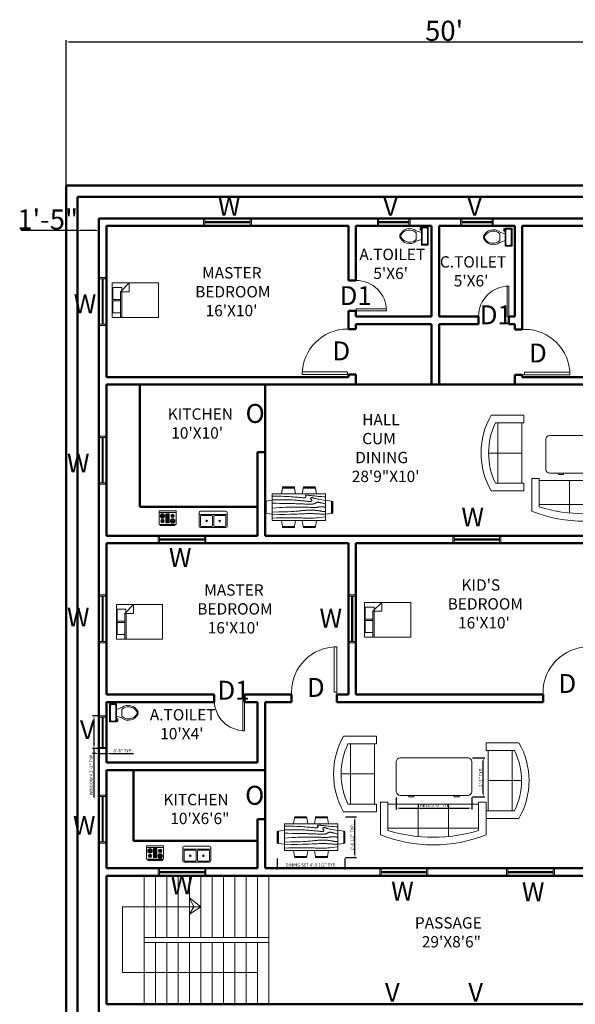
# Model space of a CAD drawing. Units: inches. Extents: x -7040 to -4088, y 6092 to 7645.
# Tile 6 of 11: x -7040 to -6599, y 6864 to 7645. Entities that reach past the tile are written whole.
import ezdxf

# ---------------------------------------------------------------- set-up
doc = ezdxf.new("R2010")
doc.units = ezdxf.units.IN
for name, color, linetype, lineweight in [('A-ANNO-DIMS', 2, 'Continuous', 18), ('A-ANNO-TEXT', 7, 'Continuous', 25), ('A-AREA-IDEN', 3, 'Continuous', 25), ('A-DOOR', 3, 'Continuous', 18), ('A-FLOR-FIXT', 9, 'Continuous', 13), ('A-FLOR-STRS', 2, 'Continuous', 18), ('A-FURN', 8, 'Continuous', 13), ('A-GLAZ', 4, 'Continuous', 18), ('A-WALL', 7, 'Continuous', 50)]:
    doc.layers.add(name, color=color, linetype=linetype, lineweight=lineweight)
doc.styles.get("Standard").update_dxf_attribs({"font": 'arial.ttf'})
doc.dimstyles.new('ISO-25', dxfattribs={"dimtxt": 2.5, "dimasz": 2.5, "dimexe": 1.25, "dimexo": 0.625, "dimtad": 1, "dimdec": 0, "dimlunit": 3, "dimtxsty": 'Standard', "dimcen": 2.5, "dimadec": 0, "dimazin": 0, "dimtfac": 1, "dimtdec": 0, "dimtmove": 0, "dimatfit": 3, "dimfxl": 1, "dimarcsym": 0})

# ---------------------------------------------------------------- blocks, each defined once
blk = doc.blocks.new('*U8')
for p, q in [((0, 0), (0, -100)), ((750, 0), (750, -100))]:
    blk.add_line(p, q)
blk.add_lwpolyline([(0, 0), (0, 750), (43.75, 750), (43.75, 0)], close=True)
blk.add_arc((0, 0), 750, 0, 90)
blk = doc.blocks.new('Bed - Queen')
for p, q in [((0, -80.00003), (0, 0)), ((0, 0), (59.99999, 0)), ((59.99999, 0), (59.99999, -80.00003)), ((0, -14.4), (44.8, -14.4)), ((44.8, -16.8), (0, -16.8)), ((7.99999, -1.2), (28.79998, -1.2)), ((7.99999, -14.4), (7.99999, -1.2)), ((28.79998, -1.2), (28.79998, -14.4)), ((31.19999, -1.2), (51.99999, -1.2)), ((31.19999, -14.4), (31.19999, -1.2)), ((59.99999, -29.6), (44.8, -14.4)), ((44.8, -14.4), (44.8, -29.6)), ((51.99999, -16.4), (46.79936, -16.4)), ((51.99999, -1.2), (51.99999, -16.4)), ((44.8, -29.6), (59.99999, -29.6)), ((59.99999, -80.00003), (0, -80.00003))]:
    blk.add_line(p, q)
blk = doc.blocks.new('Dining Set - 36 x 72 in.')
for p, q in [((-22, 27.5), (-22.1562, 26.50042)), ((-22, 27.5), (-6, 27.5)), ((-5.8437, 26.49966), (-6, 27.5)), ((6, 27.5), (5.8438, 26.50042)), ((6, 27.5), (22, 27.5)), ((22.1563, 26.49966), (22, 27.5)), ((36, 18), (-36, 18)), ((-36, 18), (-36, -18)), ((-22.2343, 26.00059), (-23.4847, 17.99762)), ((-22.2304, 26), (-5.7608, 26)), ((-5.8416, 26.5), (-22.1534, 26.5)), ((-4.5152, 17.99762), (-5.7655, 25.99926)), ((5.7657, 26.00059), (4.5153, 17.99762)), ((5.7696, 26), (22.2392, 26)), ((22.1584, 26.5), (5.8466, 26.5)), ((23.4848, 17.99762), (22.2345, 25.99926)), ((36, -18), (36, 18)), ((-45.5, 8), (-44.5004, 8.15617)), ((-45.5, 8), (-45.5, -8)), ((-44.5, -8.15843), (-44.5, 8.15338)), ((-44.0006, 8.23428), (-35.9976, 9.48474)), ((-44, 8.23041), (-44, -8.23915)), ((44.0006, 8.23428), (35.9976, 9.48474)), ((44, 8.23041), (44, -8.23915)), ((44.5, -8.15843), (44.5, 8.15338)), ((45.5, 8), (44.5005, 8.15617)), ((45.5, 8), (45.5, -8)), ((-44.4997, -8.15631), (-45.5, -8)), ((-35.9976, -9.48476), (-43.9993, -8.2345)), ((35.9976, -9.48476), (43.9993, -8.2345)), ((44.4997, -8.15631), (45.5, -8)), ((-36, -18), (36, -18)), ((-22.2343, -26.0006), (-23.4847, -17.99762)), ((-22.2304, -26), (-5.7608, -26)), ((-22, -27.5), (-22.1562, -26.50044)), ((-5.8416, -26.5), (-22.1534, -26.5)), ((-5.8437, -26.49967), (-6, -27.5)), ((-4.5152, -17.99762), (-5.7655, -25.99928)), ((5.7657, -26.0006), (4.5153, -17.99762)), ((5.7696, -26), (22.2392, -26)), ((6, -27.5), (5.8438, -26.50044)), ((22.1584, -26.5), (5.8466, -26.5)), ((22.1563, -26.49967), (22, -27.5)), ((23.4848, -17.99762), (22.2345, -25.99928)), ((-22, -27.5), (-6, -27.5)), ((6, -27.5), (22, -27.5))]:
    blk.add_line(p, q)
for points in [[(-36, 15), (-31.1772, 14.97754), (-26.8079, 14.91406), (-22.8538, 14.81543), (-19.276, 14.6875), (-16.0362, 14.53613), (-13.0957, 14.36718), (-10.4159, 14.18652), (-7.9583, 14), (-5.6904, 13.81315), (-3.6035, 13.63021), (-1.6954, 13.45508), (0.0365, 13.29166), (1.5945, 13.14388), (2.9811, 13.01562), (4.1988, 12.9108), (5.25, 12.83333), (6.1393, 12.78613), (6.8802, 12.76823), (7.4883, 12.77767), (7.9792, 12.8125), (8.3685, 12.87077), (8.6719, 12.95052), (8.9049, 13.0498), (9.0833, 13.16666), (9.2205, 13.29899), (9.3216, 13.44401), (9.3895, 13.59879), (9.4271, 13.76041), (9.4373, 13.92594), (9.4232, 14.09245), (9.3875, 14.257), (9.3333, 14.41666), (9.2638, 14.56917), (9.1836, 14.71484), (9.0975, 14.85465), (9.0104, 14.98958), (8.9272, 15.1206), (8.8529, 15.2487), (8.7922, 15.37483), (8.75, 15.5), (8.7305, 15.62467), (8.7344, 15.74739), (8.7617, 15.86621), (8.8125, 15.97916), (8.8867, 16.08431), (8.9844, 16.17968), (9.1055, 16.26334), (9.25, 16.33333), (9.4189, 16.38802), (9.6172, 16.42708), (9.8506, 16.45052), (10.125, 16.45833), (10.4463, 16.45052), (10.8203, 16.42708), (11.2529, 16.38802), (11.75, 16.33333), (12.3184, 16.26318), (12.9694, 16.17838), (13.7151, 16.07991), (14.5677, 15.96875), (15.5395, 15.84586), (16.6426, 15.71224), (17.8893, 15.56884), (19.2917, 15.41666), (20.859, 15.25667), (22.5879, 15.08984), (24.4721, 14.91715), (26.5052, 14.73958), (28.6809, 14.5581), (30.9929, 14.3737), (33.4347, 14.18733), (36, 14)], [(-36, 10), (-28.9766, 10.14274), (-23.1725, 10.20442), (-18.4241, 10.19775), (-14.5677, 10.13541), (-11.4399, 10.03011), (-8.877, 9.89453), (-6.7154, 9.74137), (-4.7917, 9.58333), (-2.9698, 9.43082), (-1.2246, 9.28515), (0.4415, 9.14534), (2.026, 9.01041), (3.5266, 8.87939), (4.9408, 8.7513), (6.266, 8.62516), (7.5, 8.5), (8.6411, 8.37549), (9.6914, 8.2539), (10.6538, 8.13818), (11.5312, 8.03125), (12.3267, 7.93603), (13.043, 7.85547), (13.6831, 7.79248), (14.25, 7.75), (14.7471, 7.7303), (15.1797, 7.73307), (15.5537, 7.75732), (15.875, 7.80208), (16.1494, 7.86637), (16.3828, 7.94922), (16.5811, 8.04964), (16.75, 8.16666), (16.8944, 8.29915), (17.0143, 8.44531), (17.1089, 8.60319), (17.1771, 8.77083), (17.218, 8.94629), (17.2305, 9.1276), (17.2137, 9.31282), (17.1667, 9.5), (17.0895, 9.6875), (16.987, 9.875), (16.8649, 10.0625), (16.7292, 10.25), (16.5856, 10.4375), (16.4401, 10.625), (16.2985, 10.8125), (16.1667, 11), (16.05, 11.18733), (15.9518, 11.3737), (15.8752, 11.5581), (15.8229, 11.73958), (15.798, 11.91715), (15.8034, 12.08984), (15.842, 12.25667), (15.9167, 12.41666), (16.0295, 12.56836), (16.1784, 12.70833), (16.3605, 12.83268), (16.5729, 12.9375), (16.8127, 13.01888), (17.0768, 13.07291), (17.3625, 13.0957), (17.6667, 13.08333), (17.9894, 13.03312), (18.3418, 12.94726), (18.7382, 12.82918), (19.1927, 12.68229), (19.7195, 12.51001), (20.3327, 12.31575), (21.0465, 12.10294), (21.875, 11.875), (22.8357, 11.63354), (23.959, 11.37304), (25.2786, 11.08618), (26.8282, 10.76562), (28.6414, 10.40405), (30.752, 9.99414), (33.1936, 9.52856), (36, 9)], [(-36, 5.5), (-30.7157, 5.3348), (-26.069, 5.20963), (-21.9946, 5.11767), (-18.4271, 5.05208), (-15.3009, 5.00602), (-12.5508, 4.97265), (-10.1112, 4.94515), (-7.9167, 4.91666), (-5.909, 4.88167), (-4.0586, 4.83984), (-2.3429, 4.79215), (-0.7396, 4.73958), (0.7739, 4.6831), (2.22, 4.6237), (3.6213, 4.56233), (5, 4.5), (6.373, 4.43782), (7.7344, 4.3776), (9.0723, 4.32129), (10.375, 4.27083), (11.6309, 4.22819), (12.8281, 4.19531), (13.9551, 4.17415), (15, 4.16666), (15.954, 4.17448), (16.819, 4.19791), (17.6001, 4.23698), (18.3021, 4.29166), (18.9299, 4.36198), (19.4883, 4.44791), (19.9823, 4.54948), (20.4167, 4.66666), (20.7969, 4.79899), (21.1302, 4.94401), (21.4245, 5.09879), (21.6875, 5.26041), (21.9271, 5.42594), (22.1511, 5.59245), (22.3672, 5.757), (22.5834, 5.91666), (22.8065, 6.06868), (23.0404, 6.21093), (23.2879, 6.34147), (23.5521, 6.45833), (23.8358, 6.55957), (24.142, 6.64323), (24.4735, 6.70735), (24.8334, 6.75), (25.2235, 6.76969), (25.642, 6.76692), (26.0858, 6.74267), (26.5521, 6.69791), (27.0379, 6.63362), (27.5404, 6.55078), (28.0565, 6.45036), (28.5834, 6.33333), (29.1242, 6.19987), (29.7071, 6.04687), (30.3661, 5.87044), (31.1354, 5.66666), (32.0493, 5.43164), (33.142, 5.16146), (34.4475, 4.85221), (36, 4.5)], [(-36, -1), (-30.7915, -0.6591), (-26.0195, -0.38216), (-21.6519, -0.16284), (-17.6563, 0.00521), (-14.0005, 0.12833), (-10.6523, 0.21289), (-7.5796, 0.26522), (-4.75, 0.29166), (-2.134, 0.29793), (0.2878, 0.28711), (2.5317, 0.26163), (4.6146, 0.22396), (6.5529, 0.17651), (8.3633, 0.12174), (10.0623, 0.06209), (11.6667, 0), (13.1899, -0.06201), (14.6341, -0.1211), (15.9982, -0.17432), (17.2813, -0.21875), (18.4823, -0.25147), (19.6003, -0.26953), (20.6343, -0.27002), (21.5834, -0.25), (22.4481, -0.20768), (23.2357, -0.14584), (23.9549, -0.06836), (24.6146, 0.02083), (25.2235, 0.11784), (25.7904, 0.21875), (26.3241, 0.31966), (26.8334, 0.41666), (27.3265, 0.50618), (27.8099, 0.58593), (28.2894, 0.65397), (28.7709, 0.70833), (29.2601, 0.74707), (29.763, 0.76823), (30.2855, 0.76985), (30.8334, 0.75), (31.4088, 0.70784), (31.9994, 0.64713), (32.589, 0.57275), (33.1615, 0.48958), (33.7008, 0.4025), (34.1908, 0.3164), (34.6153, 0.23616), (34.9584, 0.16666), (35.2099, 0.11165), (35.3848, 0.07031), (35.504, 0.04069), (35.5886, 0.02083), (35.6594, 0.00879), (35.7377, 0.0026), (35.8442, 0.00032), (36, 0)], [(-36, -6.5), (-27.1843, -6.31267), (-20.084, -6.1263), (-14.469, -5.9419), (-10.1094, -5.76042), (-6.7752, -5.58285), (-4.2363, -5.41016), (-2.2629, -5.24333), (-0.625, -5.08334), (0.8708, -4.93099), (2.2715, -4.78646), (3.5872, -4.64974), (4.8281, -4.52084), (6.0046, -4.39974), (7.127, -4.28646), (8.2053, -4.18099), (9.25, -4.08334), (10.2705, -3.99382), (11.2734, -3.91407), (12.2647, -3.84603), (13.25, -3.79167), (14.2354, -3.75293), (15.2266, -3.73177), (16.2295, -3.73015), (17.25, -3.75), (18.2912, -3.79248), (19.3451, -3.85547), (20.4009, -3.93604), (21.4479, -4.03125), (22.4754, -4.13819), (23.4727, -4.25391), (24.4289, -4.37549), (25.3334, -4.5), (26.1785, -4.62492), (26.9694, -4.74935), (27.7145, -4.87281), (28.4219, -4.99479), (29.1, -5.11483), (29.7572, -5.23242), (30.4016, -5.34709), (31.0417, -5.45834), (31.6837, -5.56437), (32.3262, -5.65821), (32.9658, -5.73153), (33.599, -5.77604), (34.2224, -5.78345), (34.8327, -5.74545), (35.4264, -5.65373), (36, -5.5)], [(-36, -10), (-26.4022, -9.81299), (-18.4675, -9.62891), (-11.9839, -9.45069), (-6.7396, -9.28125), (-2.5226, -9.12354), (0.8789, -8.98047), (3.6769, -8.85498), (6.0833, -8.75), (8.2767, -8.66765), (10.3021, -8.60677), (12.1712, -8.56543), (13.8958, -8.54167), (15.4876, -8.53353), (16.9583, -8.53907), (18.3197, -8.55632), (19.5834, -8.58334), (20.7616, -8.61841), (21.8685, -8.66081), (22.9188, -8.71004), (23.9271, -8.76563), (24.9081, -8.82707), (25.8763, -8.89388), (26.8465, -8.96558), (27.8334, -9.04167), (28.8474, -9.12118), (29.8828, -9.20117), (30.93, -9.27824), (31.9792, -9.34896), (33.0205, -9.40991), (34.0443, -9.45768), (35.0407, -9.48885), (36, -9.5)], [(-36, -14.5), (-30.0881, -14.33513), (-25.0332, -14.21224), (-20.7312, -14.12647), (-17.0781, -14.07292), (-13.97, -14.04671), (-11.3027, -14.04297), (-8.9724, -14.05681), (-6.875, -14.08334), (-4.9224, -14.11833), (-3.0905, -14.16016), (-1.3709, -14.20785), (0.2448, -14.26042), (1.7647, -14.3169), (3.1973, -14.3763), (4.5507, -14.43767), (5.8333, -14.5), (7.0554, -14.5621), (8.235, -14.62175), (9.3922, -14.67652), (10.5469, -14.72396), (11.7192, -14.76164), (12.929, -14.78711), (14.1965, -14.79794), (15.5417, -14.79167), (16.9933, -14.76424), (18.6152, -14.70508), (20.4804, -14.60197), (22.6615, -14.44271), (25.2312, -14.21509), (28.2624, -13.9069), (31.8277, -13.50594), (36, -13)]]:
    blk.add_lwpolyline(points)
blk = doc.blocks.new('Desk - 30 x 60 in.')
for p, q in [((-26.999995, 0), (26.999995, 0)), ((-29.999995, -27), (-29.999995, -3)), ((29.999995, -3), (29.999995, -27)), ((26.999995, -30), (-26.999995, -30)), ((-20.000005, -30), (-20.000005, -31)), ((-20.000005, -31), (-16.000005, -31)), ((-16.000005, -31), (-16.000005, -30)), ((15.999995, -31), (15.999995, -30)), ((19.999995, -31), (15.999995, -31)), ((19.999995, -30), (19.999995, -31))]:
    blk.add_line(p, q)
for centre, start, end in [((-26.499995, -3.5), 98.1301, 171.8699), ((26.499995, -3.5), 8.130102, 81.8699), ((-26.499995, -26.5), 188.1301, 261.8699), ((26.499995, -26.5), 278.1301, 351.8699)]:
    blk.add_arc(centre, 3.535534, start, end)
blk = doc.blocks.new('Sofa - Roundback 7 ft.')
for p, q in [((-12.00002, -32.4421), (-12.00003, -6.5971)), ((11.99997, -32.4421), (11.99998, -6.5971)), ((-36.000027, -34), (-36.000027, -11.4696)), ((-35.999844, -13.3819), (35.9998, -13.3819)), ((35.99998, -34), (35.99998, -11.4696)), ((-36.000027, -32.4421), (35.99998, -32.4421))]:
    blk.add_line(p, q)
for points in [[(-36.000027, -34), (-42.000027, -34), (-42.000027, -8)], [(41.99998, -8), (41.99998, -34), (35.99998, -34)]]:
    blk.add_lwpolyline(points)
for centre, radius, start, end in [((0, -114.25), 114.25, 68.43141, 111.5686), ((-0.00001, -127.1968), 121.1968, 72.72033, 107.2797)]:
    blk.add_arc(centre, radius, start, end)
blk = doc.blocks.new('Sofa - Roundback Loveseat 5 ft.')
for p, q in [((0, -32.44198), (0, -5.99998)), ((-24, -33.99998), (-24, -11.46958)), ((-23.9998, -13.38178), (23.99986, -13.38178)), ((24.00004, -33.99998), (24.00004, -11.46958)), ((-24, -32.44198), (24.00004, -32.44198))]:
    blk.add_line(p, q)
for points in [[(-24, -33.99998), (-30, -33.99998), (-30, -7.99998)], [(30.00004, -7.99998), (30.00004, -33.99998), (24.00004, -33.99998)]]:
    blk.add_lwpolyline(points)
for centre, radius, start, end in [((0, -60.24998), 60.24998, 60.13715, 119.8628), ((0, -61.38438), 55.38444, 64.32083, 115.6792)]:
    blk.add_arc(centre, radius, start, end)
blk = doc.blocks.new('Range-Oven - 30 in top')
for p, q in [((0, -3), (30, -3)), ((12, -6), (18, -6)), ((13, -20), (13, -6)), ((14, -6), (14, -20)), ((15, -20), (15, -6)), ((16, -6), (16, -20)), ((17, -20), (17, -6)), ((6, -24), (6, -25)), ((8, -25), (8, -24)), ((18, -20), (12, -20)), ((22, -25), (22, -24)), ((24, -24), (24, -25))]:
    blk.add_line(p, q)
for points in [[(0, -24), (0, 0), (30, 0), (30, -24)], [(12, -21), (12, -5), (18, -5), (18, -21)], [(2, -26), (2, -25), (28, -25), (28, -26)]]:
    blk.add_lwpolyline(points, close=True)
for centre, radius in [((6, -9), 4), ((6, -9), 3), ((6, -18), 3), ((6, -9), 2), ((6, -18), 2), ((6, -9), 1), ((6, -18), 1), ((24, -18), 4), ((24, -9), 3), ((24, -18), 3), ((24, -9), 2), ((24, -18), 2), ((24, -9), 1), ((24, -18), 1)]:
    blk.add_circle(centre, radius)
blk = doc.blocks.new('Sink-double - 36 in top')
for p, q in [((-18, -4), (18, -4)), ((-0.75, -18.5), (-0.75, -6.5)), ((0.75, -6.5), (0.75, -18.5))]:
    blk.add_line(p, q)
for points in [[(-16.5, 0), (16.5, 0)], [(-18, -19.5), (-18, -1.5)], [(-16.5, -18.5), (-16.5, -6.5)], [(-15.5, -5.5), (-1.75, -5.5)], [(1.75, -5.5), (15.5, -5.5)], [(16.5, -6.5), (16.5, -18.5)], [(18, -1.5), (18, -19.5)], [(16.5, -21), (-16.5, -21)], [(-1.75, -19.5), (-15.5, -19.5)], [(15.5, -19.5), (1.75, -19.5)]]:
    blk.add_lwpolyline(points)
for centre, radius in [((-8.5, -12.5), 1), ((-8.5, -12.5), 0.5), ((8.5, -12.5), 1), ((8.5, -12.5), 0.5)]:
    blk.add_circle(centre, radius)
for centre, radius, start, end in [((-16.5, -1.5), 1.5, 90, 180), ((16.5, -1.5), 1.5, 0, 90), ((-15.5, -6.5), 1, 90, 180), ((-1.75, -6.5), 1, 0, 90), ((1.75, -6.5), 1, 90, 180), ((15.5, -6.5), 1, 0, 90), ((-16.5, -19.5), 1.5, 180, 270), ((-15.5, -18.5), 1, 180, 270), ((-1.75, -18.5), 1, 270, 0), ((1.75, -18.5), 1, 180, 270), ((15.5, -18.5), 1, 270, 0), ((16.5, -19.5), 1.5, 270, 0)]:
    blk.add_arc(centre, radius, start, end)
blk = doc.blocks.new('Toilet - top')
for p, q in [((-10, -8.5), (-8, -8.5)), ((-10, -9.5), (-10, -8.5)), ((-7, -9.5), (-10, -9.5)), ((-8, -8.5), (-8, -8)), ((-7, -8), (-7, -9.5)), ((-4, -8), (-6, -14)), ((4, -8), (6, -14)), ((9.5, -6), (9.5, -2)), ((4, -14), (-4, -14))]:
    blk.add_line(p, q)
blk.add_lwpolyline([(10.5, -8), (10.5, 0), (-10.5, 0), (-10.5, -8)], close=True)
for points in [[(-9.5, -2), (-9.5, -6)], [(8.5, -1), (-8.5, -1)], [(-8.5, -7), (8.5, -7)]]:
    blk.add_lwpolyline(points)
for centre, radius, start, end in [((-8.6, -1.9), 0.884, 81.8699, 188.1301), ((-8.6, -6.1), 0.884, 171.8699, 278.1301), ((8.6, -1.9), 0.884, 351.8699, 98.1301), ((8.6, -6.1), 0.884, 261.8699, 8.1301), ((3.5, -21.6), 12.2, 141.4691, 247.9714), ((4.2, -21.8), 11.3, 136.3677, 238.9468), ((-3.5, -21.6), 12.2, 292.0284, 38.5307), ((-4.2, -21.8), 11.3, 301.053, 43.6321), ((0, -27.9), 4, 245.7318, 294.2682), ((0, -29), 4, 254.8605, 285.1395)]:
    blk.add_arc(centre, radius, start, end)
blk = doc.blocks.new('*D91')
at = {"layer": 'A-ANNO-DIMS', "color": 0, "lineweight": -2, "transparency": 16777216}
for p, q in [((-6994.03, 7487.13), (-6994.03, 7476.85)), ((-6977.03, 7487.13), (-6977.03, 7476.85)), ((-6994.03, 7478.1), (-7038.81, 7478.1)), ((-6979.53, 7478.1), (-6991.53, 7478.1))]:
    blk.add_line(p, q, dxfattribs=at)
at = {"layer": 'A-ANNO-DIMS', "color": 0, "transparency": 16777216}
for points in [[(-6991.53, 7478.52), (-6991.53, 7477.68), (-6994.03, 7478.1)], [(-6979.53, 7478.52), (-6979.53, 7477.68), (-6977.03, 7478.1)]]:
    blk.add_solid(points, dxfattribs=at)
at = {"layer": 'Defpoints', "color": 0, "transparency": 16777216}
for p in [(-6994.03, 7487.76), (-6977.03, 7487.76), (-6994.03, 7478.1)]:
    blk.add_point(p, dxfattribs=at)
at = {"layer": 'A-ANNO-DIMS', "color": 0, "transparency": 16777216, "insert": (-7017.67, 7486.89), "char_height": 2.5, "attachment_point": 5}
blk.add_mtext('{\\H6.4x;1\'-5"}', dxfattribs=at)
blk = doc.blocks.new('*D92')
at = {"layer": 'A-ANNO-DIMS', "color": 0, "lineweight": -2, "transparency": 16777216}
for p, q in [((-7003.03, 7514.38), (-7003.03, 7629.1)), ((-7000.53, 7627.85), (-6405.53, 7627.85)), ((-6403.03, 7514.38), (-6403.03, 7629.1))]:
    blk.add_line(p, q, dxfattribs=at)
at = {"layer": 'A-ANNO-DIMS', "color": 0, "transparency": 16777216}
for points in [[(-7000.53, 7628.27), (-7000.53, 7627.43), (-7003.03, 7627.85)], [(-6405.53, 7628.27), (-6405.53, 7627.43), (-6403.03, 7627.85)]]:
    blk.add_solid(points, dxfattribs=at)
at = {"layer": 'Defpoints', "color": 0, "transparency": 16777216}
for p in [(-6403.03, 7627.85), (-7003.03, 7513.76), (-6403.03, 7513.76)]:
    blk.add_point(p, dxfattribs=at)
at = {"layer": 'A-ANNO-DIMS', "color": 0, "transparency": 16777216, "insert": (-6703.03, 7636.64), "char_height": 2.5, "attachment_point": 5}
blk.add_mtext("{\\H6.4x;50'}", dxfattribs=at)
blk = doc.blocks.new('WIN-36')
for p, q in [((0, 6), (0, 0)), ((1, 6), (1, 0)), ((1, 3.5), (37, 3.5)), ((1, 3), (37, 3)), ((1, 2.5), (37, 2.5)), ((37, 6), (37, 0)), ((38, 6), (38, 0))]:
    blk.add_line(p, q)
blk = doc.blocks.new('WIN-24')
for p, q in [((0, 6), (0, 0)), ((1, 6), (1, 0)), ((1, 3.5), (25, 3.5)), ((1, 3), (25, 3)), ((1, 2.5), (25, 2.5)), ((25, 6), (25, 0)), ((26, 6), (26, 0))]:
    blk.add_line(p, q)
blk = doc.blocks.new('*D116')
at = {"layer": 'A-ANNO-DIMS', "color": 0, "lineweight": -2, "transparency": 16777216}
for p, q in [((-6977.66, 7092.76), (-6982.18, 7092.76)), ((-6980.93, 7090.26), (-6980.93, 7069.26)), ((-6977.66, 7066.76), (-6982.18, 7066.76)), ((-6980.93, 7066.76), (-6980.93, 7028.07))]:
    blk.add_line(p, q, dxfattribs=at)
at = {"layer": 'A-ANNO-DIMS', "color": 0, "transparency": 16777216}
for points in [[(-6981.35, 7090.26), (-6980.51, 7090.26), (-6980.93, 7092.76)], [(-6981.35, 7069.26), (-6980.51, 7069.26), (-6980.93, 7066.76)]]:
    blk.add_solid(points, dxfattribs=at)
at = {"layer": 'Defpoints', "color": 0, "transparency": 16777216}
for p in [(-6977.03, 7092.76), (-6980.93, 7066.76), (-6977.03, 7066.76)]:
    blk.add_point(p, dxfattribs=at)
at = {"layer": 'A-ANNO-DIMS', "color": 0, "transparency": 16777216, "insert": (-6982.85, 7046.17), "char_height": 2.5, "attachment_point": 5, "rotation": 90}
blk.add_mtext('WINDOW V 2\'-2" TYP.', dxfattribs=at)
blk = doc.blocks.new('*D117')
at = {"layer": 'A-ANNO-DIMS', "color": 0, "lineweight": -2, "transparency": 16777216}
for p, q in [((-6979.53, 7062.86), (-6982.03, 7062.86)), ((-6977.03, 7066.13), (-6977.03, 7061.61)), ((-6977.03, 7062.86), (-6971.03, 7062.86)), ((-6971.03, 7066.13), (-6971.03, 7061.61)), ((-6968.53, 7062.86), (-6949.54, 7062.86))]:
    blk.add_line(p, q, dxfattribs=at)
at = {"layer": 'A-ANNO-DIMS', "color": 0, "transparency": 16777216}
for points in [[(-6979.53, 7063.28), (-6979.53, 7062.44), (-6977.03, 7062.86)], [(-6968.53, 7063.28), (-6968.53, 7062.44), (-6971.03, 7062.86)]]:
    blk.add_solid(points, dxfattribs=at)
at = {"layer": 'Defpoints', "color": 0, "transparency": 16777216}
for p in [(-6977.03, 7066.76), (-6971.03, 7066.76), (-6971.03, 7062.86)]:
    blk.add_point(p, dxfattribs=at)
at = {"layer": 'A-ANNO-DIMS', "color": 0, "transparency": 16777216, "insert": (-6957.79, 7064.76), "char_height": 2.5, "attachment_point": 5}
blk.add_mtext('0\'-6" TYP.', dxfattribs=at)
blk = doc.blocks.new('*D142')
at = {"layer": 'A-ANNO-DIMS', "color": 0, "lineweight": -2, "transparency": 16777216}
for p, q in [((-6835.41, 6979.57), (-6835.41, 6970.91)), ((-6781.86, 6979.57), (-6781.86, 6970.91)), ((-6832.91, 6972.16), (-6784.36, 6972.16))]:
    blk.add_line(p, q, dxfattribs=at)
at = {"layer": 'A-ANNO-DIMS', "color": 0, "transparency": 16777216}
for points in [[(-6832.91, 6972.58), (-6832.91, 6971.75), (-6835.41, 6972.16)], [(-6784.36, 6972.58), (-6784.36, 6971.75), (-6781.86, 6972.16)]]:
    blk.add_solid(points, dxfattribs=at)
at = {"layer": 'Defpoints', "color": 0, "transparency": 16777216}
for p in [(-6835.41, 6980.2), (-6781.86, 6980.2), (-6781.86, 6972.16)]:
    blk.add_point(p, dxfattribs=at)
at = {"layer": 'A-ANNO-DIMS', "color": 0, "transparency": 16777216, "insert": (-6808.64, 6974.08), "char_height": 2.5, "attachment_point": 5}
blk.add_mtext('DINING SET 4\'-5 1/2" TYP.', dxfattribs=at)
blk = doc.blocks.new('*D143')
at = {"layer": 'A-ANNO-DIMS', "color": 0, "lineweight": -2, "transparency": 16777216}
for p, q in [((-6781.24, 7012.56), (-6772.58, 7012.56)), ((-6773.83, 6982.7), (-6773.83, 7010.06)), ((-6781.24, 6980.2), (-6772.58, 6980.2))]:
    blk.add_line(p, q, dxfattribs=at)
at = {"layer": 'A-ANNO-DIMS', "color": 0, "transparency": 16777216}
for points in [[(-6774.25, 7010.06), (-6773.41, 7010.06), (-6773.83, 7012.56)], [(-6774.25, 6982.7), (-6773.41, 6982.7), (-6773.83, 6980.2)]]:
    blk.add_solid(points, dxfattribs=at)
at = {"layer": 'Defpoints', "color": 0, "transparency": 16777216}
for p in [(-6781.86, 7012.56), (-6773.83, 7012.56), (-6781.86, 6980.2)]:
    blk.add_point(p, dxfattribs=at)
at = {"layer": 'A-ANNO-DIMS', "color": 0, "transparency": 16777216, "insert": (-6775.75, 6996.38), "char_height": 2.5, "attachment_point": 5, "rotation": 90}
blk.add_mtext('2\'-8 1/2" TYP.', dxfattribs=at)
blk = doc.blocks.new('*D160')
at = {"layer": 'A-ANNO-DIMS', "color": 0, "lineweight": -2, "transparency": 16777216}
for p, q in [((-6741.03, 7027.92), (-6741.03, 7018.3)), ((-6681.03, 7027.92), (-6681.03, 7018.3)), ((-6738.53, 7019.55), (-6683.53, 7019.55))]:
    blk.add_line(p, q, dxfattribs=at)
at = {"layer": 'A-ANNO-DIMS', "color": 0, "transparency": 16777216}
for points in [[(-6738.53, 7019.96), (-6738.53, 7019.13), (-6741.03, 7019.55)], [(-6683.53, 7019.96), (-6683.53, 7019.13), (-6681.03, 7019.55)]]:
    blk.add_solid(points, dxfattribs=at)
at = {"layer": 'Defpoints', "color": 0, "transparency": 16777216}
for p in [(-6741.03, 7028.55), (-6681.03, 7028.55), (-6681.03, 7019.55)]:
    blk.add_point(p, dxfattribs=at)
at = {"layer": 'A-ANNO-DIMS', "color": 0, "transparency": 16777216, "insert": (-6711.03, 7021.45), "char_height": 2.5, "attachment_point": 5}
blk.add_mtext('TABLE 5\'-0" TYP.', dxfattribs=at)
blk = doc.blocks.new('*D161')
at = {"layer": 'A-ANNO-DIMS', "color": 0, "lineweight": -2, "transparency": 16777216}
for p, q in [((-6680.41, 7059.55), (-6670.78, 7059.55)), ((-6672.03, 7031.05), (-6672.03, 7057.05)), ((-6680.41, 7028.55), (-6670.78, 7028.55))]:
    blk.add_line(p, q, dxfattribs=at)
at = {"layer": 'A-ANNO-DIMS', "color": 0, "transparency": 16777216}
for points in [[(-6672.45, 7057.05), (-6671.61, 7057.05), (-6672.03, 7059.55)], [(-6672.45, 7031.05), (-6671.61, 7031.05), (-6672.03, 7028.55)]]:
    blk.add_solid(points, dxfattribs=at)
at = {"layer": 'Defpoints', "color": 0, "transparency": 16777216}
for p in [(-6681.03, 7059.55), (-6672.03, 7059.55), (-6681.03, 7028.55)]:
    blk.add_point(p, dxfattribs=at)
at = {"layer": 'A-ANNO-DIMS', "color": 0, "transparency": 16777216, "insert": (-6673.91, 7044.05), "char_height": 2.5, "attachment_point": 5, "rotation": 90}
blk.add_mtext('2\'-7" TYP.', dxfattribs=at)

msp = doc.modelspace()

# ---------------------------------------------------------------- linework, layer by layer
at = {"layer": 'A-FLOR-STRS'}
for p, q in [((-6941.03, 6863.76), (-6941.03, 6965.76)), ((-6932.03, 6916.76), (-6932.03, 6965.76)), ((-6923.03, 6916.76), (-6923.03, 6965.76)), ((-6914.03, 6916.76), (-6914.03, 6965.76)), ((-6905.03, 6916.76), (-6905.03, 6965.76)), ((-6896.03, 6916.76), (-6896.03, 6965.76)), ((-6887.03, 6916.76), (-6887.03, 6965.76)), ((-6878.03, 6916.76), (-6878.03, 6965.76)), ((-6869.03, 6916.76), (-6869.03, 6965.76)), ((-6860.03, 6916.76), (-6860.03, 6965.76)), ((-6851.03, 6916.76), (-6851.03, 6965.76)), ((-6842.03, 6863.76), (-6842.03, 6965.76)), ((-6896.03, 6941.26), (-6905.03, 6948.34)), ((-6905.03, 6948.34), (-6901.7, 6941.26)), ((-6896.03, 6941.26), (-6958.33, 6941.26)), ((-6958.33, 6941.26), (-6958.33, 6888.95)), ((-6901.7, 6941.26), (-6905.03, 6935.38)), ((-6905.03, 6935.38), (-6896.03, 6941.26)), ((-6941.03, 6916.76), (-6842.03, 6916.76)), ((-6941.03, 6912.76), (-6842.03, 6912.76)), ((-6932.03, 6863.76), (-6932.03, 6912.76)), ((-6923.03, 6863.76), (-6923.03, 6912.76)), ((-6914.03, 6863.76), (-6914.03, 6912.76)), ((-6905.03, 6863.76), (-6905.03, 6912.76)), ((-6896.03, 6863.76), (-6896.03, 6912.76)), ((-6887.03, 6863.76), (-6887.03, 6912.76)), ((-6878.03, 6863.76), (-6878.03, 6912.76)), ((-6869.03, 6863.76), (-6869.03, 6912.76)), ((-6860.03, 6863.76), (-6860.03, 6912.76)), ((-6851.03, 6863.76), (-6851.03, 6912.76)), ((-6958.33, 6888.95), (-6851.03, 6888.95))]:
    msp.add_line(p, q, dxfattribs=at)
at = {"layer": 'A-GLAZ'}
for p, q in [((-6977.03, 7440.76), (-6971.03, 7440.76)), ((-6977.03, 7440.76), (-6971.03, 7440.76)), ((-6977.03, 7439.76), (-6971.03, 7439.76)), ((-6977.03, 7439.76), (-6971.03, 7439.76)), ((-6974.53, 7403.76), (-6974.53, 7439.76)), ((-6974.53, 7403.76), (-6974.53, 7439.76)), ((-6974.03, 7403.76), (-6974.03, 7439.76)), ((-6974.03, 7403.76), (-6974.03, 7439.76)), ((-6973.53, 7403.76), (-6973.53, 7439.76)), ((-6973.53, 7403.76), (-6973.53, 7439.76)), ((-6977.03, 7403.76), (-6971.03, 7403.76)), ((-6977.03, 7403.76), (-6971.03, 7403.76)), ((-6977.03, 7402.76), (-6971.03, 7402.76)), ((-6977.03, 7402.76), (-6971.03, 7402.76)), ((-6977.03, 7314.76), (-6971.03, 7314.76)), ((-6977.03, 7314.76), (-6971.03, 7314.76)), ((-6977.03, 7313.76), (-6971.03, 7313.76)), ((-6977.03, 7313.76), (-6971.03, 7313.76)), ((-6974.53, 7277.76), (-6974.53, 7313.76)), ((-6974.53, 7277.76), (-6974.53, 7313.76)), ((-6974.03, 7277.76), (-6974.03, 7313.76)), ((-6974.03, 7277.76), (-6974.03, 7313.76)), ((-6973.53, 7277.76), (-6973.53, 7313.76)), ((-6973.53, 7277.76), (-6973.53, 7313.76)), ((-6977.03, 7277.76), (-6971.03, 7277.76)), ((-6977.03, 7277.76), (-6971.03, 7277.76)), ((-6977.03, 7276.76), (-6971.03, 7276.76)), ((-6977.03, 7276.76), (-6971.03, 7276.76)), ((-6977.03, 7188.76), (-6971.03, 7188.76)), ((-6977.03, 7188.76), (-6971.03, 7188.76)), ((-6977.03, 7187.76), (-6971.03, 7187.76)), ((-6977.03, 7187.76), (-6971.03, 7187.76)), ((-6974.53, 7151.76), (-6974.53, 7187.76)), ((-6974.53, 7151.76), (-6974.53, 7187.76)), ((-6974.03, 7151.76), (-6974.03, 7187.76)), ((-6974.03, 7151.76), (-6974.03, 7187.76)), ((-6973.53, 7151.76), (-6973.53, 7187.76)), ((-6973.53, 7151.76), (-6973.53, 7187.76)), ((-6779.03, 7188.76), (-6773.03, 7188.76)), ((-6779.03, 7188.76), (-6773.03, 7188.76)), ((-6779.03, 7187.76), (-6773.03, 7187.76)), ((-6779.03, 7187.76), (-6773.03, 7187.76)), ((-6776.53, 7151.76), (-6776.53, 7187.76)), ((-6776.53, 7151.76), (-6776.53, 7187.76)), ((-6776.03, 7151.76), (-6776.03, 7187.76)), ((-6776.03, 7151.76), (-6776.03, 7187.76)), ((-6775.53, 7151.76), (-6775.53, 7187.76)), ((-6775.53, 7151.76), (-6775.53, 7187.76)), ((-6977.03, 7151.76), (-6971.03, 7151.76)), ((-6977.03, 7151.76), (-6971.03, 7151.76)), ((-6977.03, 7150.76), (-6971.03, 7150.76)), ((-6977.03, 7150.76), (-6971.03, 7150.76)), ((-6779.03, 7151.76), (-6773.03, 7151.76)), ((-6779.03, 7151.76), (-6773.03, 7151.76)), ((-6779.03, 7150.76), (-6773.03, 7150.76)), ((-6779.03, 7150.76), (-6773.03, 7150.76)), ((-6977.03, 7029.76), (-6971.03, 7029.76)), ((-6977.03, 7029.76), (-6971.03, 7029.76)), ((-6977.03, 7028.76), (-6971.03, 7028.76)), ((-6977.03, 7028.76), (-6971.03, 7028.76)), ((-6974.53, 6992.76), (-6974.53, 7028.76)), ((-6974.53, 6992.76), (-6974.53, 7028.76)), ((-6974.03, 6992.76), (-6974.03, 7028.76)), ((-6974.03, 6992.76), (-6974.03, 7028.76)), ((-6973.53, 6992.76), (-6973.53, 7028.76)), ((-6973.53, 6992.76), (-6973.53, 7028.76)), ((-6977.03, 6992.76), (-6971.03, 6992.76)), ((-6977.03, 6992.76), (-6971.03, 6992.76)), ((-6977.03, 6991.76), (-6971.03, 6991.76)), ((-6977.03, 6991.76), (-6971.03, 6991.76))]:
    msp.add_line(p, q, dxfattribs=at)
at = {"layer": 'A-WALL'}
for p, q in [((-7003.03, 7513.76), (-6403.03, 7513.76)), ((-7003.03, 6156.76), (-7003.03, 7513.76)), ((-6994.03, 7504.76), (-6412.03, 7504.76)), ((-6994.03, 6179.76), (-6994.03, 7504.76)), ((-6977.03, 6179.76), (-6977.03, 7487.76)), ((-6977.03, 7487.76), (-6475.03, 7487.76)), ((-6971.03, 7481.76), (-6779.03, 7481.76)), ((-6971.03, 7361.76), (-6971.03, 7481.76)), ((-6779.03, 7438.44), (-6779.03, 7481.76)), ((-6779.03, 7438.44), (-6779.03, 7481.76)), ((-6773.03, 7481.76), (-6713.03, 7481.76)), ((-6773.03, 7438.44), (-6773.03, 7481.76)), ((-6773.03, 7438.44), (-6773.03, 7481.76)), ((-6713.03, 7409.76), (-6713.03, 7481.76)), ((-6707.03, 7409.76), (-6707.03, 7481.76)), ((-6707.03, 7481.76), (-6647.03, 7481.76)), ((-6647.03, 7409.76), (-6647.03, 7481.76)), ((-6641.03, 7481.76), (-6481.03, 7481.76)), ((-6641.03, 7399.63), (-6641.03, 7481.76)), ((-6779.03, 7438.44), (-6773.03, 7438.44)), ((-6779.03, 7414.44), (-6773.03, 7414.44)), ((-6779.03, 7399.85), (-6779.03, 7414.44)), ((-6779.03, 7399.85), (-6779.03, 7414.44)), ((-6773.03, 7409.76), (-6773.03, 7414.44)), ((-6773.03, 7409.76), (-6773.03, 7414.44)), ((-6773.03, 7409.76), (-6713.03, 7409.76)), ((-6773.03, 7403.76), (-6713.03, 7403.76)), ((-6773.03, 7399.85), (-6773.03, 7403.76)), ((-6773.03, 7399.85), (-6773.03, 7403.76)), ((-6713.03, 7355.76), (-6713.03, 7403.76)), ((-6707.03, 7409.76), (-6675.72, 7409.76)), ((-6707.03, 7355.76), (-6707.03, 7403.76)), ((-6707.03, 7403.76), (-6675.72, 7403.76)), ((-6675.72, 7409.76), (-6675.72, 7403.76)), ((-6651.72, 7409.76), (-6651.72, 7403.76)), ((-6651.72, 7409.76), (-6647.03, 7409.76)), ((-6651.72, 7403.76), (-6647.03, 7403.76)), ((-6647.03, 7399.63), (-6647.03, 7403.76)), ((-6779.03, 7399.85), (-6773.03, 7399.85)), ((-6647.03, 7399.63), (-6641.03, 7399.63)), ((-6779.03, 7361.76), (-6779.03, 7363.85)), ((-6779.03, 7361.76), (-6779.03, 7363.85)), ((-6779.03, 7363.85), (-6773.03, 7363.85)), ((-6773.03, 7355.76), (-6773.03, 7363.85)), ((-6773.03, 7355.76), (-6773.03, 7363.85)), ((-6971.03, 7361.76), (-6779.03, 7361.76)), ((-6647.03, 7355.76), (-6647.03, 7363.63)), ((-6647.03, 7363.63), (-6641.03, 7363.63)), ((-6641.03, 7361.76), (-6641.03, 7363.63)), ((-6641.03, 7361.76), (-6481.03, 7361.76)), ((-6971.03, 7355.76), (-6845.03, 7355.76)), ((-6971.03, 7235.76), (-6971.03, 7355.76)), ((-6944.6, 7355.76), (-6944.6, 7258.72)), ((-6845.03, 7355.76), (-6481.03, 7355.76)), ((-6845.03, 7302.04), (-6845.03, 7355.76)), ((-6851.03, 7235.76), (-6851.03, 7302.04)), ((-6851.03, 7235.76), (-6851.03, 7302.04)), ((-6851.03, 7302.04), (-6845.03, 7302.04)), ((-6845.03, 7235.76), (-6845.03, 7302.04)), ((-6845.03, 7235.76), (-6845.03, 7302.04)), ((-6944.6, 7258.72), (-6851.03, 7258.72)), ((-6971.03, 7235.76), (-6851.03, 7235.76)), ((-6845.03, 7235.76), (-6481.03, 7235.76)), ((-6971.03, 7229.76), (-6779.03, 7229.76)), ((-6971.03, 7109.76), (-6971.03, 7229.76)), ((-6779.03, 7109.76), (-6779.03, 7229.76)), ((-6773.03, 7109.76), (-6773.03, 7229.76)), ((-6773.03, 7229.76), (-6581.03, 7229.76)), ((-6971.03, 7109.76), (-6885.42, 7109.76)), ((-6885.42, 7109.76), (-6885.42, 7103.76)), ((-6861.42, 7109.76), (-6861.42, 7103.76)), ((-6861.42, 7109.76), (-6824.2, 7109.76)), ((-6824.2, 7109.76), (-6824.2, 7103.76)), ((-6788.2, 7109.76), (-6788.2, 7103.76)), ((-6788.2, 7109.76), (-6779.03, 7109.76)), ((-6773.03, 7109.76), (-6624.57, 7109.76)), ((-6624.57, 7109.76), (-6624.57, 7103.76)), ((-6971.03, 7103.76), (-6885.42, 7103.76)), ((-6971.03, 7055.76), (-6971.03, 7103.76)), ((-6861.42, 7103.76), (-6851.03, 7103.76)), ((-6851.03, 7055.76), (-6851.03, 7103.76)), ((-6845.03, 7103.76), (-6824.2, 7103.76)), ((-6845.03, 7049.76), (-6845.03, 7103.76)), ((-6788.2, 7103.76), (-6624.57, 7103.76)), ((-6971.03, 7055.76), (-6851.03, 7055.76)), ((-6971.03, 7049.76), (-6845.03, 7049.76)), ((-6971.03, 6971.76), (-6971.03, 7049.76)), ((-6949.58, 7049.76), (-6949.58, 6993.43)), ((-6845.03, 7010.76), (-6845.03, 7049.76)), ((-6851.03, 6971.76), (-6851.03, 7010.76)), ((-6851.03, 7010.76), (-6845.03, 7010.76)), ((-6845.03, 6971.76), (-6845.03, 7010.76)), ((-6949.58, 6993.43), (-6851.03, 6993.43)), ((-6971.03, 6971.76), (-6851.03, 6971.76)), ((-6971.03, 6965.76), (-6475.03, 6965.76)), ((-6971.03, 6863.76), (-6971.03, 6965.76)), ((-6845.03, 6971.76), (-6481.03, 6971.76)), ((-6971.03, 6863.76), (-6475.03, 6863.76))]:
    msp.add_line(p, q, dxfattribs=at)

# ---------------------------------------------------------------- block references
at = {"layer": 'A-DOOR'}
for p, xscale, yscale, zscale, rotation in [((-6772.83, 7414.44), -0.0319999973918968, 0.0319999973918968, 0.0319999973918968, 270), ((-6779.64, 7363.85), 0.0480047089255457, 0.0480047089255457, 0.0480047089255457, 90), ((-6639.23, 7363.63), -0.0479999965272596, 0.0479999965272596, 0.0479999965272596, 270), ((-6861.42, 7104.99), 0.0320007809907896, 0.0320007809907896, 0.0320007809907896, 180)]:
    msp.add_blockref('*U8', p, dxfattribs=dict(at, xscale=xscale, yscale=yscale, zscale=zscale, rotation=rotation))
for p, xscale, yscale, zscale in [((-6651.72, 7409.96), -0.0319999999999955, 0.0319999999999955, 0.0319999999999955), ((-6788.2, 7111.56), -0.0480000000000005, 0.0480000000000005, 0.0480000000000005), ((-6588.57, 7111.39), -0.0480000000000005, 0.0480000000000005, 0.0480000000000005)]:
    msp.add_blockref('*U8', p, dxfattribs=dict(at, xscale=xscale, yscale=yscale, zscale=zscale))
at = {"layer": 'A-FLOR-FIXT', "xscale": 0.6837915443005316, "yscale": 0.6837915443005316, "zscale": 0.6837915443005316}
for p, rotation in [((-6715.66, 7473.66), 270), ((-6649.17, 7472.79), 270), ((-6968.48, 7095.17), 89.99999999999999)]:
    msp.add_blockref('Toilet - top', p, dxfattribs=dict(at, rotation=rotation))
at = {"layer": 'A-FLOR-FIXT'}
for name, p, xscale, yscale, zscale in [('Range-Oven - 30 in top', (-6929.24, 7255.52), 0.4479334271382261, 0.4479334271382261, 0.4479334271382261), ('Sink-double - 36 in top', (-6886.34, 7255.19), 0.6130704979608608, 0.6130704979608608, 0.6130704979608608), ('Range-Oven - 30 in top', (-6939.14, 6989.62), 0.4479334271382261, 0.4479334271382261, 0.4479334271382261), ('Sink-double - 36 in top', (-6899.29, 6989.38), 0.6130704979608608, 0.6130704979608608, 0.6130704979608608)]:
    msp.add_blockref(name, p, dxfattribs=dict(at, xscale=xscale, yscale=yscale, zscale=zscale))
at = {"layer": 'A-FURN', "xscale": 0.4580400962997241, "yscale": 0.4580400962997241, "zscale": 0.4580400962997241, "rotation": 90}
for p in [(-6966.43, 7408.95), (-6963.1, 7153.59), (-6766.13, 7155.37)]:
    msp.add_blockref('Bed - Queen', p, dxfattribs=at)
at = {"layer": 'A-FURN'}
for name, p, rotation in [('Sofa - Roundback Loveseat 5 ft.', (-6673.75, 7301.4), 89.99999999999999), ('Sofa - Roundback 7 ft.', (-6591.57, 7247.24), 180), ('Sofa - Roundback Loveseat 5 ft.', (-6790.81, 7046.62), 89.99999999999999), ('Sofa - Roundback Loveseat 5 ft.', (-6635.66, 7041.33), 270), ('Sofa - Roundback 7 ft.', (-6711.66, 6990.33), 180)]:
    msp.add_blockref(name, p, dxfattribs=dict(at, rotation=rotation))
for p in [(-6592.41, 7315.38), (-6711.03, 7059.55)]:
    msp.add_blockref('Desk - 30 x 60 in.', p, dxfattribs=at)
at = {"layer": 'A-FURN', "xscale": 0.5884256662281149, "yscale": 0.5884256662281149, "zscale": 0.5884256662281149}
for p in [(-6818.26, 7258.36), (-6808.64, 6996.38)]:
    msp.add_blockref('Dining Set - 36 x 72 in.', p, dxfattribs=at)
at = {"layer": 'A-GLAZ'}
for name, p in [('WIN-36', (-6894.03, 7481.76)), ('WIN-24', (-6690.03, 7481.76)), ('WIN-36', (-6930.03, 7229.76)), ('WIN-36', (-6696.03, 7229.76)), ('WIN-36', (-6930.03, 6965.76)), ('WIN-36', (-6753.97, 6965.76)), ('WIN-36', (-6653.49, 6965.76))]:
    msp.add_blockref(name, p, dxfattribs=at)
for p, rotation in [((-6730.03, 7487.76), 180), ((-6977.03, 7092.76), 269.9999999999962)]:
    msp.add_blockref('WIN-24', p, dxfattribs=dict(at, rotation=rotation))

# ---------------------------------------------------------------- texts
at = {"layer": 'A-ANNO-TEXT', "char_height": 15, "attachment_point": 1}
for s, insert in [('{W}', (-6882.62, 7504.84)), ('{V}', (-6751.51, 7504.8)), ('{V}', (-6684.74, 7504.8)), ('{W}', (-6997, 7427.41)), ('{D1}', (-6785.94, 7433.89)), ('{D1}', (-6674.75, 7418.65)), ('{D}', (-6791.69, 7390.02)), ('{D}', (-6635.65, 7388.34)), ('{O}', (-6860.61, 7340.34)), ('{W}', (-7002.38, 7300.98)), ('{W}', (-6689.37, 7258.13)), ('{W}', (-6921.49, 7225.99)), ('{W}', (-7002.38, 7178.72)), ('{W}', (-6801.96, 7177.74)), ('{D}', (-6811.92, 7122.83)), ('{D}', (-6612.31, 7125.94)), ('{D1}', (-6882.91, 7120.6)), ('{V}', (-6992.04, 7089.27)), ('{O}', (-6860.95, 7037.23)), ('{W}', (-6997.62, 7013.38)), ('{W}', (-6920.2, 6966.08)), ('{W}', (-6745.1, 6961.06)), ('{W}', (-6641.38, 6960.59)), ('{V}', (-6750.04, 6880.8)), ('{V}', (-6683.92, 6880.8))]:
    msp.add_mtext_dynamic_manual_height_columns(s, width=701.5203, gutter_width=12.5, heights=[0], dxfattribs=dict(at, insert=insert))
at = {"layer": 'A-AREA-IDEN', "char_height": 9, "attachment_point": 1}
for s, insert in [("{  A.TOILET\\P      5'X6'}", (-6775.74, 7463.62)), ("{  C.TOILET\\P      5'X6'}", (-6711.9, 7457.68)), ("{  MASTER\\PBEDROOM\\P   16'X10'}", (-6900.59, 7449)), ("{  KITCHEN\\P   10'X10'}", (-6927.84, 7336.92)), ('{    HALL\\P    CUM\\P  DINING\\P 28\'9"X10\'}', (-6779.07, 7332.38)), ("{     KID'S\\P BEDROOM\\P    16'X10'}", (-6703, 7201.17)), ("{  MASTER\\PBEDROOM\\P   16'X10'}", (-6898.9, 7197.2)), ("{  A.TOILET\\P     10'X4'}", (-6942.08, 7098.15)), ('{  KITCHEN\\P    10\'X6\'6"}', (-6931.36, 7030.8)), ('{ PASSAGE\\P   29\'X8\'6"}', (-6728.99, 6932.91))]:
    msp.add_mtext_dynamic_manual_height_columns(s, width=930.9751, gutter_width=12.5, heights=[0], dxfattribs=dict(at, insert=insert))

# ---------------------------------------------------------------- dimensions: what is measured, and where the dimension line sits
at = {"layer": 'A-ANNO-DIMS'}
for base, p1, p2, text, override, picture, middle in [((-6403.03, 7627.85), (-7003.03, 7513.76), (-6403.03, 7513.76), '{\\H6.4x;<>}', {"dimclrd": 0, "dimclre": 0, "dimclrt": 0}, '*D92', (-6703.03, 7636.64)), ((-6994.03, 7478.1), (-6977.03, 7487.76), (-6994.03, 7487.76), '{\\H6.4x;<>}', {"dimclrd": 0, "dimclre": 0, "dimclrt": 0}, '*D91', (-7017.67, 7486.89)), ((-6971.03, 7062.86), (-6977.03, 7066.76), (-6971.03, 7066.76), '<> TYP.', {"dimdec": 1, "dimrnd": 0, "dimzin": 1, "dimlunit": 4, "dimfrac": 2}, '*D117', (-6957.79, 7064.76)), ((-6681.03, 7019.55), (-6741.03, 7028.55), (-6681.03, 7028.55), 'TABLE <> TYP.', {"dimdec": 1, "dimrnd": 0, "dimzin": 1, "dimlunit": 4, "dimfrac": 2}, '*D160', (-6711.03, 7021.45)), ((-6781.863, 6972.1647), (-6835.4098, 6980.1968), (-6781.863, 6980.1968), 'DINING SET <> TYP.', {"dimdec": 1, "dimrnd": 0, "dimzin": 1, "dimlunit": 4, "dimfrac": 2}, '*D142', (-6808.6364, 6974.0824))]:
    dim = msp.add_linear_dim(base=base, p1=p1, p2=p2, text=text, dimstyle='ISO-25', override=override, dxfattribs=at)
    dim.commit()
    dim.dimension.update_dxf_attribs({"geometry": picture, "text_midpoint": middle})
for base, p1, p2, angle, text, picture, middle in [((-6980.93, 7066.76), (-6977.03, 7092.76), (-6977.03, 7066.76), 270, 'WINDOW V <> TYP.', '*D116', (-6982.85, 7046.17)), ((-6672.03, 7059.55), (-6681.03, 7028.55), (-6681.03, 7059.55), 90, '<> TYP.', '*D161', (-6673.91, 7044.05)), ((-6773.83, 7012.56), (-6781.86, 6980.2), (-6781.86, 7012.56), 90, '<> TYP.', '*D143', (-6775.75, 6996.38))]:
    dim = msp.add_linear_dim(base=base, p1=p1, p2=p2, angle=angle, text=text, dimstyle='ISO-25', override={"dimdec": 1, "dimrnd": 0, "dimzin": 1, "dimlunit": 4, "dimfrac": 2}, dxfattribs=at)
    dim.commit()
    dim.dimension.update_dxf_attribs({"geometry": picture, "text_midpoint": middle})

doc.saveas('drawing.dxf')
